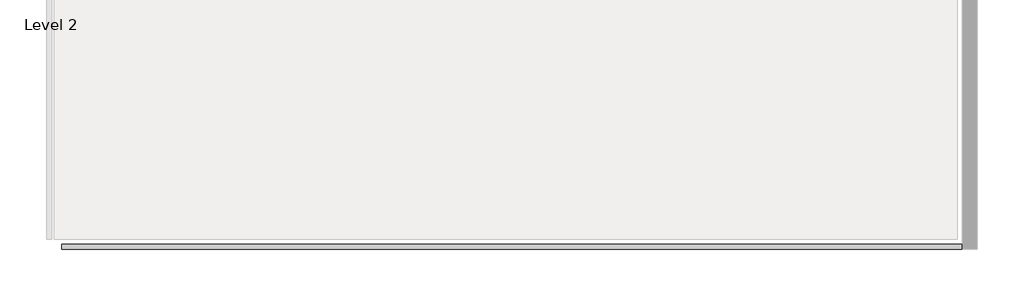
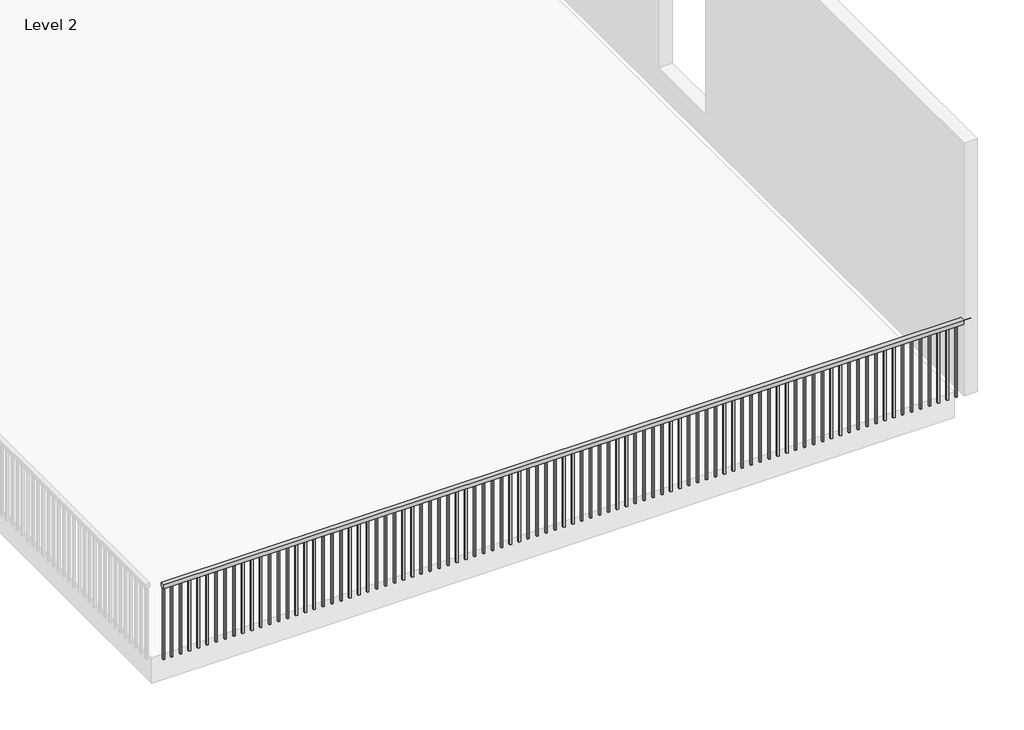
# One storey, part 2 of 4: 1 railing.
"""IFC4 building model written with IfcOpenShell, lengths in millimetres."""

from ifc_helpers import new_model, si_unit, frame, origin, place, context, project, spatial, polyline, outline, extrude, element, save

model = new_model("IFC4")

# Units and contexts
model_context = context("Model", 3, world=origin())
ifc_project = project(units=[si_unit("LENGTHUNIT", "METRE", prefix="MILLI")], contexts=[model_context])

# Site, building, storey
site = spatial("IfcSite", under=ifc_project)
building = spatial("IfcBuilding", under=site)
storey = spatial("IfcBuildingStorey", under=building, Name="Level 2", Elevation=3048.0)

# Railing
placement = place(None, origin())
element("IfcRailing", 1, ObjectType="Handrail - Rectangular", at=placement, inside=storey, context=model_context, shape_type="SweptSolid", body=[
    extrude(outline(polyline([(-11958.860887, -4709.4089531), (-11958.860887, -4658.6089531), (-2764.060887, -4658.6089531), (-2764.060887, -4709.4089531), (-11958.860887, -4709.4089531)])), frame((0.0, 0.0, 3911.6), z_axis=(0.0, 0.0, 1.0), x_axis=(1.0, 0.0, 0.0)), (0.0, 0.0, 1.0), 50.8),
    extrude(outline(polyline([(-2824.385887, -4693.5339531), (-2824.385887, -4674.4839531), (-2805.335887, -4674.4839531), (-2805.335887, -4693.5339531), (-2824.385887, -4693.5339531)])), frame((0.0, 0.0, 3048.0), z_axis=(0.0, 0.0, 1.0), x_axis=(1.0, 0.0, 0.0)), (0.0, 0.0, 1.0), 863.6),
    extrude(outline(polyline([(-2925.985887, -4693.5339531), (-2925.985887, -4674.4839531), (-2906.935887, -4674.4839531), (-2906.935887, -4693.5339531), (-2925.985887, -4693.5339531)])), frame((0.0, 0.0, 3048.0), z_axis=(0.0, 0.0, 1.0), x_axis=(1.0, 0.0, 0.0)), (0.0, 0.0, 1.0), 863.6),
    extrude(outline(polyline([(-3027.585887, -4693.5339531), (-3027.585887, -4674.4839531), (-3008.535887, -4674.4839531), (-3008.535887, -4693.5339531), (-3027.585887, -4693.5339531)])), frame((0.0, 0.0, 3048.0), z_axis=(0.0, 0.0, 1.0), x_axis=(1.0, 0.0, 0.0)), (0.0, 0.0, 1.0), 863.6),
    extrude(outline(polyline([(-3129.185887, -4693.5339531), (-3129.185887, -4674.4839531), (-3110.135887, -4674.4839531), (-3110.135887, -4693.5339531), (-3129.185887, -4693.5339531)])), frame((0.0, 0.0, 3048.0), z_axis=(0.0, 0.0, 1.0), x_axis=(1.0, 0.0, 0.0)), (0.0, 0.0, 1.0), 863.6),
    extrude(outline(polyline([(-3230.785887, -4693.5339531), (-3230.785887, -4674.4839531), (-3211.735887, -4674.4839531), (-3211.735887, -4693.5339531), (-3230.785887, -4693.5339531)])), frame((0.0, 0.0, 3048.0), z_axis=(0.0, 0.0, 1.0), x_axis=(1.0, 0.0, 0.0)), (0.0, 0.0, 1.0), 863.6),
    extrude(outline(polyline([(-3332.385887, -4693.5339531), (-3332.385887, -4674.4839531), (-3313.335887, -4674.4839531), (-3313.335887, -4693.5339531), (-3332.385887, -4693.5339531)])), frame((0.0, 0.0, 3048.0), z_axis=(0.0, 0.0, 1.0), x_axis=(1.0, 0.0, 0.0)), (0.0, 0.0, 1.0), 863.6),
    extrude(outline(polyline([(-3433.985887, -4693.5339531), (-3433.985887, -4674.4839531), (-3414.935887, -4674.4839531), (-3414.935887, -4693.5339531), (-3433.985887, -4693.5339531)])), frame((0.0, 0.0, 3048.0), z_axis=(0.0, 0.0, 1.0), x_axis=(1.0, 0.0, 0.0)), (0.0, 0.0, 1.0), 863.6),
    extrude(outline(polyline([(-3535.585887, -4693.5339531), (-3535.585887, -4674.4839531), (-3516.535887, -4674.4839531), (-3516.535887, -4693.5339531), (-3535.585887, -4693.5339531)])), frame((0.0, 0.0, 3048.0), z_axis=(0.0, 0.0, 1.0), x_axis=(1.0, 0.0, 0.0)), (0.0, 0.0, 1.0), 863.6),
    extrude(outline(polyline([(-3637.185887, -4693.5339531), (-3637.185887, -4674.4839531), (-3618.135887, -4674.4839531), (-3618.135887, -4693.5339531), (-3637.185887, -4693.5339531)])), frame((0.0, 0.0, 3048.0), z_axis=(0.0, 0.0, 1.0), x_axis=(1.0, 0.0, 0.0)), (0.0, 0.0, 1.0), 863.6),
    extrude(outline(polyline([(-3738.785887, -4693.5339531), (-3738.785887, -4674.4839531), (-3719.735887, -4674.4839531), (-3719.735887, -4693.5339531), (-3738.785887, -4693.5339531)])), frame((0.0, 0.0, 3048.0), z_axis=(0.0, 0.0, 1.0), x_axis=(1.0, 0.0, 0.0)), (0.0, 0.0, 1.0), 863.6),
    extrude(outline(polyline([(-3840.385887, -4693.5339531), (-3840.385887, -4674.4839531), (-3821.335887, -4674.4839531), (-3821.335887, -4693.5339531), (-3840.385887, -4693.5339531)])), frame((0.0, 0.0, 3048.0), z_axis=(0.0, 0.0, 1.0), x_axis=(1.0, 0.0, 0.0)), (0.0, 0.0, 1.0), 863.6),
    extrude(outline(polyline([(-3941.985887, -4693.5339531), (-3941.985887, -4674.4839531), (-3922.935887, -4674.4839531), (-3922.935887, -4693.5339531), (-3941.985887, -4693.5339531)])), frame((0.0, 0.0, 3048.0), z_axis=(0.0, 0.0, 1.0), x_axis=(1.0, 0.0, 0.0)), (0.0, 0.0, 1.0), 863.6),
    extrude(outline(polyline([(-4043.585887, -4693.5339531), (-4043.585887, -4674.4839531), (-4024.535887, -4674.4839531), (-4024.535887, -4693.5339531), (-4043.585887, -4693.5339531)])), frame((0.0, 0.0, 3048.0), z_axis=(0.0, 0.0, 1.0), x_axis=(1.0, 0.0, 0.0)), (0.0, 0.0, 1.0), 863.6),
    extrude(outline(polyline([(-4145.185887, -4693.5339531), (-4145.185887, -4674.4839531), (-4126.135887, -4674.4839531), (-4126.135887, -4693.5339531), (-4145.185887, -4693.5339531)])), frame((0.0, 0.0, 3048.0), z_axis=(0.0, 0.0, 1.0), x_axis=(1.0, 0.0, 0.0)), (0.0, 0.0, 1.0), 863.6),
    extrude(outline(polyline([(-4246.785887, -4693.5339531), (-4246.785887, -4674.4839531), (-4227.735887, -4674.4839531), (-4227.735887, -4693.5339531), (-4246.785887, -4693.5339531)])), frame((0.0, 0.0, 3048.0), z_axis=(0.0, 0.0, 1.0), x_axis=(1.0, 0.0, 0.0)), (0.0, 0.0, 1.0), 863.6),
    extrude(outline(polyline([(-4348.385887, -4693.5339531), (-4348.385887, -4674.4839531), (-4329.335887, -4674.4839531), (-4329.335887, -4693.5339531), (-4348.385887, -4693.5339531)])), frame((0.0, 0.0, 3048.0), z_axis=(0.0, 0.0, 1.0), x_axis=(1.0, 0.0, 0.0)), (0.0, 0.0, 1.0), 863.6),
    extrude(outline(polyline([(-4449.985887, -4693.5339531), (-4449.985887, -4674.4839531), (-4430.935887, -4674.4839531), (-4430.935887, -4693.5339531), (-4449.985887, -4693.5339531)])), frame((0.0, 0.0, 3048.0), z_axis=(0.0, 0.0, 1.0), x_axis=(1.0, 0.0, 0.0)), (0.0, 0.0, 1.0), 863.6),
    extrude(outline(polyline([(-4551.585887, -4693.5339531), (-4551.585887, -4674.4839531), (-4532.535887, -4674.4839531), (-4532.535887, -4693.5339531), (-4551.585887, -4693.5339531)])), frame((0.0, 0.0, 3048.0), z_axis=(0.0, 0.0, 1.0), x_axis=(1.0, 0.0, 0.0)), (0.0, 0.0, 1.0), 863.6),
    extrude(outline(polyline([(-4653.185887, -4693.5339531), (-4653.185887, -4674.4839531), (-4634.135887, -4674.4839531), (-4634.135887, -4693.5339531), (-4653.185887, -4693.5339531)])), frame((0.0, 0.0, 3048.0), z_axis=(0.0, 0.0, 1.0), x_axis=(1.0, 0.0, 0.0)), (0.0, 0.0, 1.0), 863.6),
    extrude(outline(polyline([(-4754.785887, -4693.5339531), (-4754.785887, -4674.4839531), (-4735.735887, -4674.4839531), (-4735.735887, -4693.5339531), (-4754.785887, -4693.5339531)])), frame((0.0, 0.0, 3048.0), z_axis=(0.0, 0.0, 1.0), x_axis=(1.0, 0.0, 0.0)), (0.0, 0.0, 1.0), 863.6),
    extrude(outline(polyline([(-4856.385887, -4693.5339531), (-4856.385887, -4674.4839531), (-4837.335887, -4674.4839531), (-4837.335887, -4693.5339531), (-4856.385887, -4693.5339531)])), frame((0.0, 0.0, 3048.0), z_axis=(0.0, 0.0, 1.0), x_axis=(1.0, 0.0, 0.0)), (0.0, 0.0, 1.0), 863.6),
    extrude(outline(polyline([(-4957.985887, -4693.5339531), (-4957.985887, -4674.4839531), (-4938.935887, -4674.4839531), (-4938.935887, -4693.5339531), (-4957.985887, -4693.5339531)])), frame((0.0, 0.0, 3048.0), z_axis=(0.0, 0.0, 1.0), x_axis=(1.0, 0.0, 0.0)), (0.0, 0.0, 1.0), 863.6),
    extrude(outline(polyline([(-5059.585887, -4693.5339531), (-5059.585887, -4674.4839531), (-5040.535887, -4674.4839531), (-5040.535887, -4693.5339531), (-5059.585887, -4693.5339531)])), frame((0.0, 0.0, 3048.0), z_axis=(0.0, 0.0, 1.0), x_axis=(1.0, 0.0, 0.0)), (0.0, 0.0, 1.0), 863.6),
    extrude(outline(polyline([(-5161.185887, -4693.5339531), (-5161.185887, -4674.4839531), (-5142.135887, -4674.4839531), (-5142.135887, -4693.5339531), (-5161.185887, -4693.5339531)])), frame((0.0, 0.0, 3048.0), z_axis=(0.0, 0.0, 1.0), x_axis=(1.0, 0.0, 0.0)), (0.0, 0.0, 1.0), 863.6),
    extrude(outline(polyline([(-5262.785887, -4693.5339531), (-5262.785887, -4674.4839531), (-5243.735887, -4674.4839531), (-5243.735887, -4693.5339531), (-5262.785887, -4693.5339531)])), frame((0.0, 0.0, 3048.0), z_axis=(0.0, 0.0, 1.0), x_axis=(1.0, 0.0, 0.0)), (0.0, 0.0, 1.0), 863.6),
    extrude(outline(polyline([(-5364.385887, -4693.5339531), (-5364.385887, -4674.4839531), (-5345.335887, -4674.4839531), (-5345.335887, -4693.5339531), (-5364.385887, -4693.5339531)])), frame((0.0, 0.0, 3048.0), z_axis=(0.0, 0.0, 1.0), x_axis=(1.0, 0.0, 0.0)), (0.0, 0.0, 1.0), 863.6),
    extrude(outline(polyline([(-5465.985887, -4693.5339531), (-5465.985887, -4674.4839531), (-5446.935887, -4674.4839531), (-5446.935887, -4693.5339531), (-5465.985887, -4693.5339531)])), frame((0.0, 0.0, 3048.0), z_axis=(0.0, 0.0, 1.0), x_axis=(1.0, 0.0, 0.0)), (0.0, 0.0, 1.0), 863.6),
    extrude(outline(polyline([(-5567.585887, -4693.5339531), (-5567.585887, -4674.4839531), (-5548.535887, -4674.4839531), (-5548.535887, -4693.5339531), (-5567.585887, -4693.5339531)])), frame((0.0, 0.0, 3048.0), z_axis=(0.0, 0.0, 1.0), x_axis=(1.0, 0.0, 0.0)), (0.0, 0.0, 1.0), 863.6),
    extrude(outline(polyline([(-5669.185887, -4693.5339531), (-5669.185887, -4674.4839531), (-5650.135887, -4674.4839531), (-5650.135887, -4693.5339531), (-5669.185887, -4693.5339531)])), frame((0.0, 0.0, 3048.0), z_axis=(0.0, 0.0, 1.0), x_axis=(1.0, 0.0, 0.0)), (0.0, 0.0, 1.0), 863.6),
    extrude(outline(polyline([(-5770.785887, -4693.5339531), (-5770.785887, -4674.4839531), (-5751.735887, -4674.4839531), (-5751.735887, -4693.5339531), (-5770.785887, -4693.5339531)])), frame((0.0, 0.0, 3048.0), z_axis=(0.0, 0.0, 1.0), x_axis=(1.0, 0.0, 0.0)), (0.0, 0.0, 1.0), 863.6),
    extrude(outline(polyline([(-5872.385887, -4693.5339531), (-5872.385887, -4674.4839531), (-5853.335887, -4674.4839531), (-5853.335887, -4693.5339531), (-5872.385887, -4693.5339531)])), frame((0.0, 0.0, 3048.0), z_axis=(0.0, 0.0, 1.0), x_axis=(1.0, 0.0, 0.0)), (0.0, 0.0, 1.0), 863.6),
    extrude(outline(polyline([(-5973.985887, -4693.5339531), (-5973.985887, -4674.4839531), (-5954.935887, -4674.4839531), (-5954.935887, -4693.5339531), (-5973.985887, -4693.5339531)])), frame((0.0, 0.0, 3048.0), z_axis=(0.0, 0.0, 1.0), x_axis=(1.0, 0.0, 0.0)), (0.0, 0.0, 1.0), 863.6),
    extrude(outline(polyline([(-6075.585887, -4693.5339531), (-6075.585887, -4674.4839531), (-6056.535887, -4674.4839531), (-6056.535887, -4693.5339531), (-6075.585887, -4693.5339531)])), frame((0.0, 0.0, 3048.0), z_axis=(0.0, 0.0, 1.0), x_axis=(1.0, 0.0, 0.0)), (0.0, 0.0, 1.0), 863.6),
    extrude(outline(polyline([(-6177.185887, -4693.5339531), (-6177.185887, -4674.4839531), (-6158.135887, -4674.4839531), (-6158.135887, -4693.5339531), (-6177.185887, -4693.5339531)])), frame((0.0, 0.0, 3048.0), z_axis=(0.0, 0.0, 1.0), x_axis=(1.0, 0.0, 0.0)), (0.0, 0.0, 1.0), 863.6),
    extrude(outline(polyline([(-6278.785887, -4693.5339531), (-6278.785887, -4674.4839531), (-6259.735887, -4674.4839531), (-6259.735887, -4693.5339531), (-6278.785887, -4693.5339531)])), frame((0.0, 0.0, 3048.0), z_axis=(0.0, 0.0, 1.0), x_axis=(1.0, 0.0, 0.0)), (0.0, 0.0, 1.0), 863.6),
    extrude(outline(polyline([(-6380.385887, -4693.5339531), (-6380.385887, -4674.4839531), (-6361.335887, -4674.4839531), (-6361.335887, -4693.5339531), (-6380.385887, -4693.5339531)])), frame((0.0, 0.0, 3048.0), z_axis=(0.0, 0.0, 1.0), x_axis=(1.0, 0.0, 0.0)), (0.0, 0.0, 1.0), 863.6),
    extrude(outline(polyline([(-6481.985887, -4693.5339531), (-6481.985887, -4674.4839531), (-6462.935887, -4674.4839531), (-6462.935887, -4693.5339531), (-6481.985887, -4693.5339531)])), frame((0.0, 0.0, 3048.0), z_axis=(0.0, 0.0, 1.0), x_axis=(1.0, 0.0, 0.0)), (0.0, 0.0, 1.0), 863.6),
    extrude(outline(polyline([(-6583.585887, -4693.5339531), (-6583.585887, -4674.4839531), (-6564.535887, -4674.4839531), (-6564.535887, -4693.5339531), (-6583.585887, -4693.5339531)])), frame((0.0, 0.0, 3048.0), z_axis=(0.0, 0.0, 1.0), x_axis=(1.0, 0.0, 0.0)), (0.0, 0.0, 1.0), 863.6),
    extrude(outline(polyline([(-6685.185887, -4693.5339531), (-6685.185887, -4674.4839531), (-6666.135887, -4674.4839531), (-6666.135887, -4693.5339531), (-6685.185887, -4693.5339531)])), frame((0.0, 0.0, 3048.0), z_axis=(0.0, 0.0, 1.0), x_axis=(1.0, 0.0, 0.0)), (0.0, 0.0, 1.0), 863.6),
    extrude(outline(polyline([(-6786.785887, -4693.5339531), (-6786.785887, -4674.4839531), (-6767.735887, -4674.4839531), (-6767.735887, -4693.5339531), (-6786.785887, -4693.5339531)])), frame((0.0, 0.0, 3048.0), z_axis=(0.0, 0.0, 1.0), x_axis=(1.0, 0.0, 0.0)), (0.0, 0.0, 1.0), 863.6),
    extrude(outline(polyline([(-6888.385887, -4693.5339531), (-6888.385887, -4674.4839531), (-6869.335887, -4674.4839531), (-6869.335887, -4693.5339531), (-6888.385887, -4693.5339531)])), frame((0.0, 0.0, 3048.0), z_axis=(0.0, 0.0, 1.0), x_axis=(1.0, 0.0, 0.0)), (0.0, 0.0, 1.0), 863.6),
    extrude(outline(polyline([(-6989.985887, -4693.5339531), (-6989.985887, -4674.4839531), (-6970.935887, -4674.4839531), (-6970.935887, -4693.5339531), (-6989.985887, -4693.5339531)])), frame((0.0, 0.0, 3048.0), z_axis=(0.0, 0.0, 1.0), x_axis=(1.0, 0.0, 0.0)), (0.0, 0.0, 1.0), 863.6),
    extrude(outline(polyline([(-7091.585887, -4693.5339531), (-7091.585887, -4674.4839531), (-7072.535887, -4674.4839531), (-7072.535887, -4693.5339531), (-7091.585887, -4693.5339531)])), frame((0.0, 0.0, 3048.0), z_axis=(0.0, 0.0, 1.0), x_axis=(1.0, 0.0, 0.0)), (0.0, 0.0, 1.0), 863.6),
    extrude(outline(polyline([(-7193.185887, -4693.5339531), (-7193.185887, -4674.4839531), (-7174.135887, -4674.4839531), (-7174.135887, -4693.5339531), (-7193.185887, -4693.5339531)])), frame((0.0, 0.0, 3048.0), z_axis=(0.0, 0.0, 1.0), x_axis=(1.0, 0.0, 0.0)), (0.0, 0.0, 1.0), 863.6),
    extrude(outline(polyline([(-7294.785887, -4693.5339531), (-7294.785887, -4674.4839531), (-7275.735887, -4674.4839531), (-7275.735887, -4693.5339531), (-7294.785887, -4693.5339531)])), frame((0.0, 0.0, 3048.0), z_axis=(0.0, 0.0, 1.0), x_axis=(1.0, 0.0, 0.0)), (0.0, 0.0, 1.0), 863.6),
    extrude(outline(polyline([(-7396.385887, -4693.5339531), (-7396.385887, -4674.4839531), (-7377.335887, -4674.4839531), (-7377.335887, -4693.5339531), (-7396.385887, -4693.5339531)])), frame((0.0, 0.0, 3048.0), z_axis=(0.0, 0.0, 1.0), x_axis=(1.0, 0.0, 0.0)), (0.0, 0.0, 1.0), 863.6),
    extrude(outline(polyline([(-7497.985887, -4693.5339531), (-7497.985887, -4674.4839531), (-7478.935887, -4674.4839531), (-7478.935887, -4693.5339531), (-7497.985887, -4693.5339531)])), frame((0.0, 0.0, 3048.0), z_axis=(0.0, 0.0, 1.0), x_axis=(1.0, 0.0, 0.0)), (0.0, 0.0, 1.0), 863.6),
    extrude(outline(polyline([(-7599.585887, -4693.5339531), (-7599.585887, -4674.4839531), (-7580.535887, -4674.4839531), (-7580.535887, -4693.5339531), (-7599.585887, -4693.5339531)])), frame((0.0, 0.0, 3048.0), z_axis=(0.0, 0.0, 1.0), x_axis=(1.0, 0.0, 0.0)), (0.0, 0.0, 1.0), 863.6),
    extrude(outline(polyline([(-7701.185887, -4693.5339531), (-7701.185887, -4674.4839531), (-7682.135887, -4674.4839531), (-7682.135887, -4693.5339531), (-7701.185887, -4693.5339531)])), frame((0.0, 0.0, 3048.0), z_axis=(0.0, 0.0, 1.0), x_axis=(1.0, 0.0, 0.0)), (0.0, 0.0, 1.0), 863.6),
    extrude(outline(polyline([(-7802.785887, -4693.5339531), (-7802.785887, -4674.4839531), (-7783.735887, -4674.4839531), (-7783.735887, -4693.5339531), (-7802.785887, -4693.5339531)])), frame((0.0, 0.0, 3048.0), z_axis=(0.0, 0.0, 1.0), x_axis=(1.0, 0.0, 0.0)), (0.0, 0.0, 1.0), 863.6),
    extrude(outline(polyline([(-7904.385887, -4693.5339531), (-7904.385887, -4674.4839531), (-7885.335887, -4674.4839531), (-7885.335887, -4693.5339531), (-7904.385887, -4693.5339531)])), frame((0.0, 0.0, 3048.0), z_axis=(0.0, 0.0, 1.0), x_axis=(1.0, 0.0, 0.0)), (0.0, 0.0, 1.0), 863.6),
    extrude(outline(polyline([(-8005.985887, -4693.5339531), (-8005.985887, -4674.4839531), (-7986.935887, -4674.4839531), (-7986.935887, -4693.5339531), (-8005.985887, -4693.5339531)])), frame((0.0, 0.0, 3048.0), z_axis=(0.0, 0.0, 1.0), x_axis=(1.0, 0.0, 0.0)), (0.0, 0.0, 1.0), 863.6),
    extrude(outline(polyline([(-8107.585887, -4693.5339531), (-8107.585887, -4674.4839531), (-8088.535887, -4674.4839531), (-8088.535887, -4693.5339531), (-8107.585887, -4693.5339531)])), frame((0.0, 0.0, 3048.0), z_axis=(0.0, 0.0, 1.0), x_axis=(1.0, 0.0, 0.0)), (0.0, 0.0, 1.0), 863.6),
    extrude(outline(polyline([(-8209.185887, -4693.5339531), (-8209.185887, -4674.4839531), (-8190.135887, -4674.4839531), (-8190.135887, -4693.5339531), (-8209.185887, -4693.5339531)])), frame((0.0, 0.0, 3048.0), z_axis=(0.0, 0.0, 1.0), x_axis=(1.0, 0.0, 0.0)), (0.0, 0.0, 1.0), 863.6),
    extrude(outline(polyline([(-8310.785887, -4693.5339531), (-8310.785887, -4674.4839531), (-8291.735887, -4674.4839531), (-8291.735887, -4693.5339531), (-8310.785887, -4693.5339531)])), frame((0.0, 0.0, 3048.0), z_axis=(0.0, 0.0, 1.0), x_axis=(1.0, 0.0, 0.0)), (0.0, 0.0, 1.0), 863.6),
    extrude(outline(polyline([(-8412.385887, -4693.5339531), (-8412.385887, -4674.4839531), (-8393.335887, -4674.4839531), (-8393.335887, -4693.5339531), (-8412.385887, -4693.5339531)])), frame((0.0, 0.0, 3048.0), z_axis=(0.0, 0.0, 1.0), x_axis=(1.0, 0.0, 0.0)), (0.0, 0.0, 1.0), 863.6),
    extrude(outline(polyline([(-8513.985887, -4693.5339531), (-8513.985887, -4674.4839531), (-8494.935887, -4674.4839531), (-8494.935887, -4693.5339531), (-8513.985887, -4693.5339531)])), frame((0.0, 0.0, 3048.0), z_axis=(0.0, 0.0, 1.0), x_axis=(1.0, 0.0, 0.0)), (0.0, 0.0, 1.0), 863.6),
    extrude(outline(polyline([(-8615.585887, -4693.5339531), (-8615.585887, -4674.4839531), (-8596.535887, -4674.4839531), (-8596.535887, -4693.5339531), (-8615.585887, -4693.5339531)])), frame((0.0, 0.0, 3048.0), z_axis=(0.0, 0.0, 1.0), x_axis=(1.0, 0.0, 0.0)), (0.0, 0.0, 1.0), 863.6),
    extrude(outline(polyline([(-8717.185887, -4693.5339531), (-8717.185887, -4674.4839531), (-8698.135887, -4674.4839531), (-8698.135887, -4693.5339531), (-8717.185887, -4693.5339531)])), frame((0.0, 0.0, 3048.0), z_axis=(0.0, 0.0, 1.0), x_axis=(1.0, 0.0, 0.0)), (0.0, 0.0, 1.0), 863.6),
    extrude(outline(polyline([(-8818.785887, -4693.5339531), (-8818.785887, -4674.4839531), (-8799.735887, -4674.4839531), (-8799.735887, -4693.5339531), (-8818.785887, -4693.5339531)])), frame((0.0, 0.0, 3048.0), z_axis=(0.0, 0.0, 1.0), x_axis=(1.0, 0.0, 0.0)), (0.0, 0.0, 1.0), 863.6),
    extrude(outline(polyline([(-8920.385887, -4693.5339531), (-8920.385887, -4674.4839531), (-8901.335887, -4674.4839531), (-8901.335887, -4693.5339531), (-8920.385887, -4693.5339531)])), frame((0.0, 0.0, 3048.0), z_axis=(0.0, 0.0, 1.0), x_axis=(1.0, 0.0, 0.0)), (0.0, 0.0, 1.0), 863.6),
    extrude(outline(polyline([(-9021.985887, -4693.5339531), (-9021.985887, -4674.4839531), (-9002.935887, -4674.4839531), (-9002.935887, -4693.5339531), (-9021.985887, -4693.5339531)])), frame((0.0, 0.0, 3048.0), z_axis=(0.0, 0.0, 1.0), x_axis=(1.0, 0.0, 0.0)), (0.0, 0.0, 1.0), 863.6),
    extrude(outline(polyline([(-9123.585887, -4693.5339531), (-9123.585887, -4674.4839531), (-9104.535887, -4674.4839531), (-9104.535887, -4693.5339531), (-9123.585887, -4693.5339531)])), frame((0.0, 0.0, 3048.0), z_axis=(0.0, 0.0, 1.0), x_axis=(1.0, 0.0, 0.0)), (0.0, 0.0, 1.0), 863.6),
    extrude(outline(polyline([(-9225.185887, -4693.5339531), (-9225.185887, -4674.4839531), (-9206.135887, -4674.4839531), (-9206.135887, -4693.5339531), (-9225.185887, -4693.5339531)])), frame((0.0, 0.0, 3048.0), z_axis=(0.0, 0.0, 1.0), x_axis=(1.0, 0.0, 0.0)), (0.0, 0.0, 1.0), 863.6),
    extrude(outline(polyline([(-9326.785887, -4693.5339531), (-9326.785887, -4674.4839531), (-9307.735887, -4674.4839531), (-9307.735887, -4693.5339531), (-9326.785887, -4693.5339531)])), frame((0.0, 0.0, 3048.0), z_axis=(0.0, 0.0, 1.0), x_axis=(1.0, 0.0, 0.0)), (0.0, 0.0, 1.0), 863.6),
    extrude(outline(polyline([(-9428.385887, -4693.5339531), (-9428.385887, -4674.4839531), (-9409.335887, -4674.4839531), (-9409.335887, -4693.5339531), (-9428.385887, -4693.5339531)])), frame((0.0, 0.0, 3048.0), z_axis=(0.0, 0.0, 1.0), x_axis=(1.0, 0.0, 0.0)), (0.0, 0.0, 1.0), 863.6),
    extrude(outline(polyline([(-9529.985887, -4693.5339531), (-9529.985887, -4674.4839531), (-9510.935887, -4674.4839531), (-9510.935887, -4693.5339531), (-9529.985887, -4693.5339531)])), frame((0.0, 0.0, 3048.0), z_axis=(0.0, 0.0, 1.0), x_axis=(1.0, 0.0, 0.0)), (0.0, 0.0, 1.0), 863.6),
    extrude(outline(polyline([(-9631.585887, -4693.5339531), (-9631.585887, -4674.4839531), (-9612.535887, -4674.4839531), (-9612.535887, -4693.5339531), (-9631.585887, -4693.5339531)])), frame((0.0, 0.0, 3048.0), z_axis=(0.0, 0.0, 1.0), x_axis=(1.0, 0.0, 0.0)), (0.0, 0.0, 1.0), 863.6),
    extrude(outline(polyline([(-9733.185887, -4693.5339531), (-9733.185887, -4674.4839531), (-9714.135887, -4674.4839531), (-9714.135887, -4693.5339531), (-9733.185887, -4693.5339531)])), frame((0.0, 0.0, 3048.0), z_axis=(0.0, 0.0, 1.0), x_axis=(1.0, 0.0, 0.0)), (0.0, 0.0, 1.0), 863.6),
    extrude(outline(polyline([(-9834.785887, -4693.5339531), (-9834.785887, -4674.4839531), (-9815.735887, -4674.4839531), (-9815.735887, -4693.5339531), (-9834.785887, -4693.5339531)])), frame((0.0, 0.0, 3048.0), z_axis=(0.0, 0.0, 1.0), x_axis=(1.0, 0.0, 0.0)), (0.0, 0.0, 1.0), 863.6),
    extrude(outline(polyline([(-9936.385887, -4693.5339531), (-9936.385887, -4674.4839531), (-9917.335887, -4674.4839531), (-9917.335887, -4693.5339531), (-9936.385887, -4693.5339531)])), frame((0.0, 0.0, 3048.0), z_axis=(0.0, 0.0, 1.0), x_axis=(1.0, 0.0, 0.0)), (0.0, 0.0, 1.0), 863.6),
    extrude(outline(polyline([(-10037.985887, -4693.5339531), (-10037.985887, -4674.4839531), (-10018.935887, -4674.4839531), (-10018.935887, -4693.5339531), (-10037.985887, -4693.5339531)])), frame((0.0, 0.0, 3048.0), z_axis=(0.0, 0.0, 1.0), x_axis=(1.0, 0.0, 0.0)), (0.0, 0.0, 1.0), 863.6),
    extrude(outline(polyline([(-10139.585887, -4693.5339531), (-10139.585887, -4674.4839531), (-10120.535887, -4674.4839531), (-10120.535887, -4693.5339531), (-10139.585887, -4693.5339531)])), frame((0.0, 0.0, 3048.0), z_axis=(0.0, 0.0, 1.0), x_axis=(1.0, 0.0, 0.0)), (0.0, 0.0, 1.0), 863.6),
    extrude(outline(polyline([(-10241.185887, -4693.5339531), (-10241.185887, -4674.4839531), (-10222.135887, -4674.4839531), (-10222.135887, -4693.5339531), (-10241.185887, -4693.5339531)])), frame((0.0, 0.0, 3048.0), z_axis=(0.0, 0.0, 1.0), x_axis=(1.0, 0.0, 0.0)), (0.0, 0.0, 1.0), 863.6),
    extrude(outline(polyline([(-10342.785887, -4693.5339531), (-10342.785887, -4674.4839531), (-10323.735887, -4674.4839531), (-10323.735887, -4693.5339531), (-10342.785887, -4693.5339531)])), frame((0.0, 0.0, 3048.0), z_axis=(0.0, 0.0, 1.0), x_axis=(1.0, 0.0, 0.0)), (0.0, 0.0, 1.0), 863.6),
    extrude(outline(polyline([(-10444.385887, -4693.5339531), (-10444.385887, -4674.4839531), (-10425.335887, -4674.4839531), (-10425.335887, -4693.5339531), (-10444.385887, -4693.5339531)])), frame((0.0, 0.0, 3048.0), z_axis=(0.0, 0.0, 1.0), x_axis=(1.0, 0.0, 0.0)), (0.0, 0.0, 1.0), 863.6),
    extrude(outline(polyline([(-10545.985887, -4693.5339531), (-10545.985887, -4674.4839531), (-10526.935887, -4674.4839531), (-10526.935887, -4693.5339531), (-10545.985887, -4693.5339531)])), frame((0.0, 0.0, 3048.0), z_axis=(0.0, 0.0, 1.0), x_axis=(1.0, 0.0, 0.0)), (0.0, 0.0, 1.0), 863.6),
    extrude(outline(polyline([(-10647.585887, -4693.5339531), (-10647.585887, -4674.4839531), (-10628.535887, -4674.4839531), (-10628.535887, -4693.5339531), (-10647.585887, -4693.5339531)])), frame((0.0, 0.0, 3048.0), z_axis=(0.0, 0.0, 1.0), x_axis=(1.0, 0.0, 0.0)), (0.0, 0.0, 1.0), 863.6),
    extrude(outline(polyline([(-10749.185887, -4693.5339531), (-10749.185887, -4674.4839531), (-10730.135887, -4674.4839531), (-10730.135887, -4693.5339531), (-10749.185887, -4693.5339531)])), frame((0.0, 0.0, 3048.0), z_axis=(0.0, 0.0, 1.0), x_axis=(1.0, 0.0, 0.0)), (0.0, 0.0, 1.0), 863.6),
    extrude(outline(polyline([(-10850.785887, -4693.5339531), (-10850.785887, -4674.4839531), (-10831.735887, -4674.4839531), (-10831.735887, -4693.5339531), (-10850.785887, -4693.5339531)])), frame((0.0, 0.0, 3048.0), z_axis=(0.0, 0.0, 1.0), x_axis=(1.0, 0.0, 0.0)), (0.0, 0.0, 1.0), 863.6),
    extrude(outline(polyline([(-10952.385887, -4693.5339531), (-10952.385887, -4674.4839531), (-10933.335887, -4674.4839531), (-10933.335887, -4693.5339531), (-10952.385887, -4693.5339531)])), frame((0.0, 0.0, 3048.0), z_axis=(0.0, 0.0, 1.0), x_axis=(1.0, 0.0, 0.0)), (0.0, 0.0, 1.0), 863.6),
    extrude(outline(polyline([(-11053.985887, -4693.5339531), (-11053.985887, -4674.4839531), (-11034.935887, -4674.4839531), (-11034.935887, -4693.5339531), (-11053.985887, -4693.5339531)])), frame((0.0, 0.0, 3048.0), z_axis=(0.0, 0.0, 1.0), x_axis=(1.0, 0.0, 0.0)), (0.0, 0.0, 1.0), 863.6),
    extrude(outline(polyline([(-11155.585887, -4693.5339531), (-11155.585887, -4674.4839531), (-11136.535887, -4674.4839531), (-11136.535887, -4693.5339531), (-11155.585887, -4693.5339531)])), frame((0.0, 0.0, 3048.0), z_axis=(0.0, 0.0, 1.0), x_axis=(1.0, 0.0, 0.0)), (0.0, 0.0, 1.0), 863.6),
    extrude(outline(polyline([(-11257.185887, -4693.5339531), (-11257.185887, -4674.4839531), (-11238.135887, -4674.4839531), (-11238.135887, -4693.5339531), (-11257.185887, -4693.5339531)])), frame((0.0, 0.0, 3048.0), z_axis=(0.0, 0.0, 1.0), x_axis=(1.0, 0.0, 0.0)), (0.0, 0.0, 1.0), 863.6),
    extrude(outline(polyline([(-11358.785887, -4693.5339531), (-11358.785887, -4674.4839531), (-11339.735887, -4674.4839531), (-11339.735887, -4693.5339531), (-11358.785887, -4693.5339531)])), frame((0.0, 0.0, 3048.0), z_axis=(0.0, 0.0, 1.0), x_axis=(1.0, 0.0, 0.0)), (0.0, 0.0, 1.0), 863.6),
    extrude(outline(polyline([(-11460.385887, -4693.5339531), (-11460.385887, -4674.4839531), (-11441.335887, -4674.4839531), (-11441.335887, -4693.5339531), (-11460.385887, -4693.5339531)])), frame((0.0, 0.0, 3048.0), z_axis=(0.0, 0.0, 1.0), x_axis=(1.0, 0.0, 0.0)), (0.0, 0.0, 1.0), 863.6),
    extrude(outline(polyline([(-11561.985887, -4693.5339531), (-11561.985887, -4674.4839531), (-11542.935887, -4674.4839531), (-11542.935887, -4693.5339531), (-11561.985887, -4693.5339531)])), frame((0.0, 0.0, 3048.0), z_axis=(0.0, 0.0, 1.0), x_axis=(1.0, 0.0, 0.0)), (0.0, 0.0, 1.0), 863.6),
    extrude(outline(polyline([(-11663.585887, -4693.5339531), (-11663.585887, -4674.4839531), (-11644.535887, -4674.4839531), (-11644.535887, -4693.5339531), (-11663.585887, -4693.5339531)])), frame((0.0, 0.0, 3048.0), z_axis=(0.0, 0.0, 1.0), x_axis=(1.0, 0.0, 0.0)), (0.0, 0.0, 1.0), 863.6),
    extrude(outline(polyline([(-11765.185887, -4693.5339531), (-11765.185887, -4674.4839531), (-11746.135887, -4674.4839531), (-11746.135887, -4693.5339531), (-11765.185887, -4693.5339531)])), frame((0.0, 0.0, 3048.0), z_axis=(0.0, 0.0, 1.0), x_axis=(1.0, 0.0, 0.0)), (0.0, 0.0, 1.0), 863.6),
    extrude(outline(polyline([(-11866.785887, -4693.5339531), (-11866.785887, -4674.4839531), (-11847.735887, -4674.4839531), (-11847.735887, -4693.5339531), (-11866.785887, -4693.5339531)])), frame((0.0, 0.0, 3048.0), z_axis=(0.0, 0.0, 1.0), x_axis=(1.0, 0.0, 0.0)), (0.0, 0.0, 1.0), 863.6),
    extrude(outline(polyline([(-2783.110887, -4693.5339531), (-2783.110887, -4674.4839531), (-2764.060887, -4674.4839531), (-2764.060887, -4693.5339531), (-2783.110887, -4693.5339531)])), frame((0.0, 0.0, 3048.0), z_axis=(0.0, 0.0, 1.0), x_axis=(1.0, 0.0, 0.0)), (0.0, 0.0, 1.0), 863.6),
    extrude(outline(polyline([(-11958.860887, -4693.5339531), (-11958.860887, -4674.4839531), (-11939.810887, -4674.4839531), (-11939.810887, -4693.5339531), (-11958.860887, -4693.5339531)])), frame((0.0, 0.0, 3048.0), z_axis=(0.0, 0.0, 1.0), x_axis=(1.0, 0.0, 0.0)), (0.0, 0.0, 1.0), 863.6),
])

save(model, "model.ifc")

# Revit data of these elements
# Type "Handrail - Rectangular"
#   Assembly Code = "C2010400"
#   built-in parameter 1008612 = 0.0416667 (stored number, unit not read)
#   built-in parameter 1008611 = 0.0416667 (stored number, unit not read)
#   built-in parameter 1008609 = 0.333333 (stored number, unit not read)
#   built-in parameter 1008604 = 0.166667 (stored number, unit not read)
#   built-in parameter 1008603 = 0.166667 (stored number, unit not read)
#   Railing Height = 3' - 0"
#   built-in parameter 1008630 = 2
#   built-in parameter 1008610 = 2
#   built-in parameter 1008618 = Baluster - Square : 3/4"
# Element 1 (IfcRailing, "Handrail - Rectangular")
#   Phase Created = New Construction
